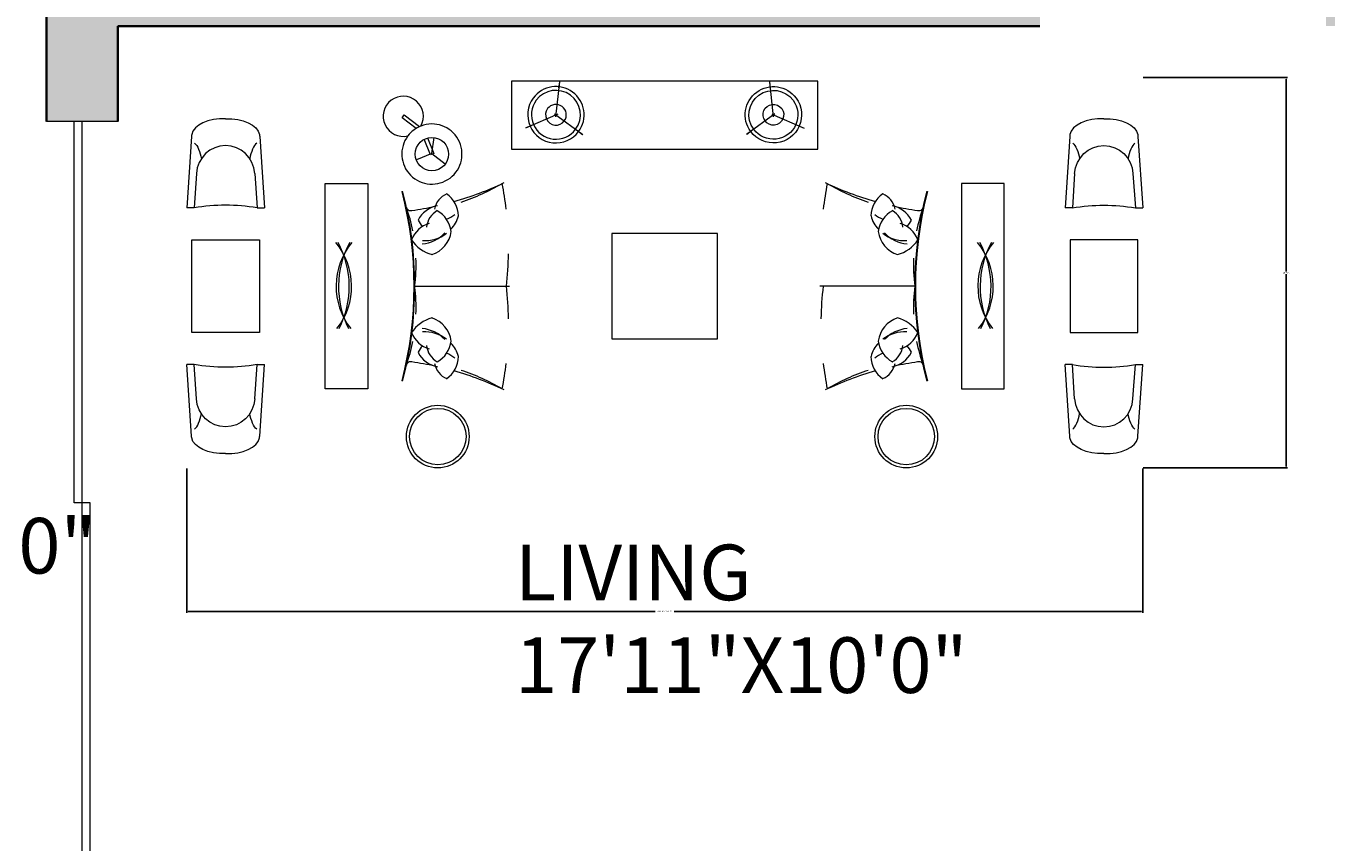
# Model space of a CAD drawing. Units: inches. Extents: x 2540 to 3167, y 3083 to 4007.
# Tile 4 of 15: x 2634 to 2798, y 3313 to 3416. Entities that reach past the tile are written whole.
import ezdxf

# ---------------------------------------------------------------- set-up
doc = ezdxf.new("R2010")
doc.units = ezdxf.units.IN
doc.set_wipeout_variables(frame=1)
for name, color, linetype, lineweight in [('A-ANNO-DIMS', 2, 'Continuous', 18), ('A-AREA-IDEN', 7, 'Continuous', 18), ('A-DOOR', 4, 'Continuous', 18), ('A-FURN', 8, 'Continuous', 13)]:
    doc.layers.add(name, color=color, linetype=linetype, lineweight=lineweight)
doc.layers.add('A-WALL', color=143, linetype='Continuous', lineweight=35, true_color=0x7aafdf)
doc.layers.add('A-WALL-PATT', color=143, linetype='Continuous', lineweight=13, true_color=0x7aafdf)
doc.styles.get("Standard").update_dxf_attribs({"font": 'arial.ttf'})
doc.dimstyles.get("Standard").update_dxf_attribs({"dimtxt": 0.18, "dimasz": 0.18, "dimexe": 0.18, "dimexo": 0.0625, "dimgap": 0.09, "dimtad": 0, "dimtih": 1, "dimtoh": 1, "dimdec": 4, "dimzin": 0, "dimdsep": 46, "dimtxsty": 'Standard', "dimcen": 0.09, "dimadec": 0, "dimazin": 0, "dimtfac": 1, "dimtdec": 4, "dimtofl": 0, "dimtmove": 0, "dimatfit": 3, "dimfxl": 1, "dimtolj": 1, "dimtzin": 0, "dimarcsym": 0})

# ---------------------------------------------------------------- blocks, each defined once
blk = doc.blocks.new('A$C5805318C')
at = {"linetype": 'ByBlock'}
for p, q in [((1718, 2794), (1735, 2817)), ((1718, 2794), (1735, 2817)), ((1735, 2817), (1857, 2723)), ((1735, 2817), (1857, 2723)), ((1829, 2708), (1718, 2794)), ((1829, 2708), (1718, 2794)), ((1945, 2497), (1893, 2622)), ((1945, 2497), (1893, 2622)), ((1919, 2633), (1971, 2508)), ((1919, 2633), (1971, 2508)), ((1955, 2509), (1973, 2636)), ((1955, 2509), (1973, 2636)), ((1955, 2509), (1831, 2459)), ((1955, 2509), (1831, 2459)), ((1971, 2508), (1945, 2497)), ((1971, 2508), (1945, 2497)), ((1955, 2509), (2060, 2427)), ((1955, 2509), (2060, 2427))]:
    blk.add_line(p, q, dxfattribs=at)
for p, q in [((38, 2645), (0, 2075)), ((582, 2645), (620, 2075)), ((7041, 2645), (7003, 2075)), ((7585, 2645), (7623, 2075)), ((77, 2348), (59, 2075)), ((543, 2348), (561, 2075)), ((7080, 2348), (7062, 2075)), ((7545, 2348), (7564, 2075)), ((59, 2075), (0, 2075)), ((561, 2075), (620, 2075)), ((7062, 2075), (7003, 2075)), ((7564, 2075), (7623, 2075)), ((59, 824), (0, 824)), ((38, 254), (0, 824)), ((77, 551), (59, 824)), ((543, 551), (561, 824)), ((561, 824), (620, 824)), ((582, 254), (620, 824)), ((7062, 824), (7003, 824)), ((7041, 254), (7003, 824)), ((7080, 551), (7062, 824)), ((7545, 551), (7564, 824)), ((7564, 824), (7623, 824)), ((7585, 254), (7623, 824))]:
    blk.add_line(p, q)
blk.add_circle((1955, 2504), 133, dxfattribs=at)
blk.add_circle((1955, 2504), 133, dxfattribs=at)
for centre, radius in [((2002, 250), 250), ((2002, 250), 225), ((5737, 250), 250), ((5737, 250), 225)]:
    blk.add_circle(centre, radius)
for centre, radius, start, end in [((1727, 2805), 160, 331.0509, 282.9948), ((1955, 2504), 240, 111.272, 142.7738), ((1955, 2504), 240, 111.272, 142.7738)]:
    blk.add_arc(centre, radius, start, end, dxfattribs=at)
for points in [[(310, 2784), (175, 2792), (54, 2736), (40, 2660), (39, 2654), (38, 2649), (38, 2643)], [(310, 2784), (445, 2792), (566, 2736), (580, 2660), (581, 2654), (582, 2649), (582, 2643)], [(7313, 2784), (7178, 2792), (7057, 2736), (7042, 2660), (7041, 2654), (7041, 2649), (7041, 2643)], [(7313, 2784), (7448, 2792), (7569, 2736), (7583, 2660), (7584, 2654), (7585, 2649), (7585, 2643)], [(310, 116), (175, 108), (54, 163), (40, 240), (39, 245), (38, 251), (38, 256)], [(310, 116), (445, 108), (566, 163), (580, 240), (581, 245), (582, 251), (582, 256)], [(7313, 116), (7178, 108), (7057, 163), (7042, 240), (7041, 245), (7041, 251), (7041, 256)], [(7313, 116), (7448, 108), (7569, 163), (7583, 240), (7584, 245), (7585, 251), (7585, 256)]]:
    blk.add_open_spline(points, degree=3, knots=[0, 0, 0, 0, 1, 1, 1, 2, 2, 2, 2])
for points in [[(62, 2590), (86, 2572), (108, 2522), (117, 2466)], [(310, 2572), (188, 2572), (86, 2474), (77, 2348)], [(543, 2348), (534, 2474), (433, 2572), (310, 2572)], [(558, 2590), (535, 2572), (512, 2522), (503, 2466)], [(7065, 2590), (7088, 2572), (7110, 2522), (7119, 2466)], [(7080, 2348), (7089, 2474), (7190, 2572), (7313, 2572)], [(7313, 2572), (7435, 2572), (7537, 2474), (7545, 2348)], [(7561, 2590), (7537, 2572), (7515, 2522), (7506, 2466)], [(310, 2096), (226, 2096), (142, 2089), (59, 2075)], [(561, 2075), (478, 2089), (394, 2096), (310, 2096)], [(7062, 2075), (7145, 2089), (7229, 2096), (7313, 2096)], [(7313, 2096), (7397, 2096), (7481, 2089), (7564, 2075)], [(310, 804), (226, 804), (142, 810), (59, 824)], [(561, 824), (478, 810), (394, 804), (310, 804)], [(7062, 824), (7145, 810), (7229, 804), (7313, 804)], [(7313, 804), (7397, 804), (7481, 810), (7564, 824)], [(310, 328), (188, 328), (86, 425), (77, 551)], [(543, 551), (534, 425), (433, 328), (310, 328)], [(7080, 551), (7089, 425), (7190, 328), (7313, 328)], [(7313, 328), (7435, 328), (7537, 425), (7545, 551)], [(62, 310), (86, 327), (108, 378), (117, 434)], [(558, 310), (535, 327), (512, 378), (503, 434)], [(7065, 310), (7088, 327), (7110, 378), (7119, 434)], [(7561, 310), (7537, 327), (7515, 378), (7506, 434)]]:
    blk.add_open_spline(points, degree=3)
for points in [[(2561, 3114), (2561, 2514), (5061, 2514), (5061, 3114)], [(1474, 600), (1074, 600), (1074, 2300), (1474, 2300)], [(2575, 1450), (2574, 1519), (2572, 1654), (2567, 1805), (2559, 1944), (2549, 2088), (2540, 2188), (2531, 2276), (2527, 2314), (1674, 2200), (1674, 1450), (1674, 699), (2527, 585), (2531, 623), (2540, 712), (2549, 811), (2559, 956), (2567, 1094), (2572, 1246), (2574, 1380)], [(5048, 1450), (5048, 1519), (5051, 1654), (5056, 1805), (5064, 1944), (5074, 2088), (5083, 2188), (5091, 2276), (5096, 2314), (5949, 2200), (5949, 1450), (5949, 699), (5096, 585), (5091, 623), (5083, 712), (5074, 811), (5064, 956), (5056, 1094), (5051, 1246), (5048, 1380)], [(6149, 600), (6549, 600), (6549, 2300), (6149, 2300)], [(3361, 1000), (4261, 1000), (4261, 1900), (3361, 1900)], [(610, 1050), (10, 1050), (10, 1850), (610, 1850)], [(7013, 1050), (7613, 1050), (7613, 1850), (7013, 1850)]]:
    blk.add_wipeout(points, dxfattribs=at)
for p, q in [((2943, 2802), (2974, 3081)), ((2968, 3032), (2974, 3078)), ((4680, 2802), (4649, 3081)), ((4654, 3032), (4649, 3078)), ((2958, 2823), (2701, 2710)), ((2932, 2826), (3159, 2659)), ((4690, 2826), (4464, 2659)), ((4665, 2823), (4922, 2710)), ((2746, 2730), (2704, 2712)), ((4877, 2730), (4919, 2712)), ((3119, 2688), (3156, 2661)), ((4504, 2688), (4467, 2661))]:
    blk.add_line(p, q, dxfattribs=at)
for p, q in [((1817, 1450), (2575, 1450)), ((5805, 1450), (5048, 1450))]:
    blk.add_line(p, q)
for points in [[(2591, 3084), (2591, 2544), (5031, 2544), (5031, 3084)], [(1444, 630), (1104, 630), (1104, 2270), (1444, 2270)], [(6179, 630), (6519, 630), (6519, 2270), (6179, 2270)], [(3391, 1030), (4231, 1030), (4231, 1870), (3391, 1870)], [(580, 1080), (40, 1080), (40, 1820), (580, 1820)], [(7043, 1080), (7583, 1080), (7583, 1820), (7043, 1820)]]:
    blk.add_lwpolyline(points, close=True, dxfattribs=at)
for centre, radius, start, end in [((1955, 2504), 240, 142.7738, 111.272), ((-1206, 1450), 3024, 345.5057, 14.4943), ((2141, 2032), 169, 113.788, 168.6748), ((1945, 2005), 222, 1.4651, 55.0097), ((1435, 4574), 2546, 285.8776, 295.5087), ((6188, 4574), 2546, 244.4913, 254.1224), ((5678, 2005), 222, 124.9903, 178.5349), ((5482, 2032), 169, 11.3252, 66.212), ((8829, 1450), 3024, 165.5057, 194.4943), ((1785, 2087), 34.6, 193.5328, 287.2771), ((1435, 4574), 2546, 278.134, 282.3755), ((2038, 1878), 217, 100.5196, 152.9581), ((5585, 1878), 217, 27.0419, 79.4804), ((6188, 4574), 2546, 257.6245, 261.866), ((5838, 2087), 34.6, 252.7229, 346.4672), ((2095, 2106), 282, 207.4684, 220.0792), ((2081, 1906), 169, 119.788, 174.6748), ((1889, 1858), 222, 7.4651, 61.0097), ((1947, 2064), 226, 314.9669, 346.4215), ((5676, 2064), 226, 193.5785, 225.0331), ((5734, 1858), 222, 118.9903, 172.5349), ((5542, 1906), 169, 5.3252, 60.212), ((5528, 2106), 282, 319.9208, 332.5316), ((1996, 1742), 217, 106.5196, 158.9581), ((1885, 1917), 226, 288.0023, 352.4215), ((5738, 1917), 226, 187.5785, 251.9977), ((5627, 1742), 217, 21.0419, 73.4804), ((769, 1450), 546, 321.7197, 39.6872), ((1737, 1450), 546, 140.3128, 218.2803), ((564, 1447), 732, 332.7542, 28.6527), ((1942, 1447), 732, 151.3473, 207.2458), ((2028, 1975), 282, 213.4684, 255.3384), ((5595, 1975), 282, 284.6616, 326.5316), ((5885, 1450), 546, 321.7197, 39.6872), ((6854, 1450), 546, 140.3128, 218.2803), ((5681, 1447), 732, 332.7542, 28.6527), ((7058, 1447), 732, 151.3473, 207.2458), ((2028, 924), 282, 104.6616, 146.5316), ((1885, 982), 226, 7.5785, 71.9977), ((5738, 982), 226, 108.0023, 172.4215), ((5595, 924), 282, 33.4684, 75.3384), ((1996, 1158), 217, 201.0419, 253.4804), ((5627, 1158), 217, 286.5196, 338.9581), ((2095, 793), 282, 139.9208, 152.5316), ((2081, 993), 169, 185.3252, 240.212), ((1889, 1041), 222, 298.9903, 352.5349), ((1947, 836), 226, 13.5785, 45.0331), ((5676, 836), 226, 134.9669, 166.4215), ((5734, 1041), 222, 187.4651, 241.0097), ((5542, 993), 169, 299.788, 354.6748), ((5528, 793), 282, 27.4684, 40.0792), ((1785, 813), 34.6, 72.7229, 166.4672), ((1435, -1675), 2546, 77.6245, 81.866), ((2038, 1021), 217, 207.0419, 259.4804), ((2141, 867), 169, 191.3252, 246.212), ((1945, 894), 222, 304.9903, 358.5349), ((5678, 894), 222, 181.4651, 235.0097), ((5482, 867), 169, 293.788, 348.6748), ((5585, 1021), 217, 280.5196, 332.9581), ((6188, -1675), 2546, 98.134, 102.3755), ((5838, 813), 34.6, 13.5328, 107.2771), ((1435, -1675), 2546, 64.4913, 74.1224), ((6188, -1675), 2546, 105.8776, 115.5087)]:
    blk.add_arc(centre, radius, start, end, dxfattribs=at)
for centre, radius, start, end in [((-1206, 1450), 3019, 345.5057, 14.4943), ((1640, 3765), 1733, 288.4757, 300.3241), ((-91, 1753), 2657, 6.7363, 11.1857), ((7714, 1753), 2657, 168.8143, 173.2637), ((5982, 3765), 1733, 239.6759, 251.5243), ((8829, 1450), 3019, 165.5057, 194.4943), ((477, 1627), 1352, 11.274, 19.5243), ((7146, 1627), 1352, 160.4757, 168.726), ((1964, 2245), 282, 292.5627, 307.9208), ((5659, 2245), 282, 232.0792, 247.4373), ((1853, 2068), 282, 275.0195, 316.8895), ((1899, 2095), 282, 266.0508, 307.9208), ((5723, 2095), 282, 232.0792, 273.9492), ((5769, 2068), 282, 223.1105, 264.9805), ((477, 1627), 1352, 352.4802, 2.0119), ((-91, 1753), 2657, 353.4417, 359.0402), ((7146, 1627), 1352, 177.9881, 187.5198), ((477, 1273), 1352, 357.9881, 7.5198), ((-91, 1146), 2657, 0.9598, 6.5583), ((7714, 1146), 2657, 173.4417, 179.0402), ((7146, 1273), 1352, 172.4802, 182.0119), ((1853, 831), 282, 43.1105, 84.9805), ((1899, 804), 282, 52.0792, 93.9492), ((5723, 804), 282, 86.0508, 127.9208), ((5769, 831), 282, 95.0195, 136.8895), ((477, 1273), 1352, 340.4757, 348.726), ((7146, 1273), 1352, 191.274, 199.5243), ((1964, 654), 282, 52.0792, 67.4373), ((-91, 1146), 2657, 348.8143, 353.2637), ((7714, 1146), 2657, 186.7363, 191.1857), ((5659, 654), 282, 112.5627, 127.9208), ((1640, -865), 1733, 59.6759, 71.5243), ((5982, -865), 1733, 108.4757, 120.3241)]:
    blk.add_arc(centre, radius, start, end)
for major_axis, start_param, end_param in [((-159, 159), 3.292387, 6.433979), ((-138, 138), 3.292387, 6.433979), ((-159, 159), 0.150794, 3.292387), ((-138, 138), 0.150794, 3.292387), ((-58.4, 58.4), 0.150794, 3.292387), ((-58.4, 58.4), 3.292387, 6.433979)]:
    blk.add_ellipse((2944, 2817), major_axis=major_axis, ratio=1, start_param=start_param, end_param=end_param, dxfattribs=at)
at = {"linetype": 'ByBlock', "extrusion": (0, 0, -1)}
for major_axis, start_param, end_param in [((159, 159), 3.292387, 6.433979), ((138, 138), 3.292387, 6.433979), ((159, 159), 0.150794, 3.292387), ((138, 138), 0.150794, 3.292387), ((-58.4, 58.4), 4.863183, 8.004776), ((-58.4, 58.4), 1.72159, 4.863183)]:
    blk.add_ellipse((4678, 2817), major_axis=major_axis, ratio=1, start_param=start_param, end_param=end_param, dxfattribs=at)
blk = doc.blocks.new('DOOR-SLIDING-96IN')
for p, q in [((9, 96), (0, 96)), ((3.5, 48), (3.5, 96)), ((4.5, 0), (4.5, 96)), ((5.5, 48), (3.5, 48)), ((5.5, 0), (5.5, 48)), ((9, 0), (0, 0))]:
    blk.add_line(p, q)
blk = doc.blocks.new('*D39')
at = {"layer": 'A-ANNO-DIMS', "color": 0, "lineweight": -2, "transparency": 16777216}
for p, q in [((2654.16, 3360.01), (2654.16, 3341.85)), ((2774.46, 3360.01), (2774.46, 3341.85)), ((2654.34, 3342.03), (2713.12, 3342.03)), ((2774.28, 3342.03), (2715.49, 3342.03))]:
    blk.add_line(p, q, dxfattribs=at)
at = {"layer": 'A-ANNO-DIMS', "color": 0, "transparency": 16777216}
for points in [[(2654.34, 3342.06), (2654.34, 3342), (2654.16, 3342.03)], [(2774.28, 3342.06), (2774.28, 3342), (2774.46, 3342.03)]]:
    blk.add_solid(points, dxfattribs=at)
at = {"layer": 'Defpoints', "color": 0, "transparency": 16777216}
for p in [(2654.16, 3360.08), (2774.46, 3360.08), (2774.46, 3342.03)]:
    blk.add_point(p, dxfattribs=at)
at = {"layer": 'A-ANNO-DIMS', "color": 0, "transparency": 16777216, "insert": (2714.31, 3342.03), "char_height": 0.18, "attachment_point": 5}
blk.add_mtext('\\A1;SEATING 120 TYP.', dxfattribs=at)
blk = doc.blocks.new('*D40')
at = {"layer": 'A-ANNO-DIMS', "color": 0, "lineweight": -2, "transparency": 16777216}
for p, q in [((2774.52, 3409.21), (2792.68, 3409.21)), ((2792.5, 3409.03), (2792.5, 3384.83)), ((2792.5, 3360.26), (2792.5, 3384.46)), ((2774.52, 3360.08), (2792.68, 3360.08))]:
    blk.add_line(p, q, dxfattribs=at)
at = {"layer": 'A-ANNO-DIMS', "color": 0, "transparency": 16777216}
for points in [[(2792.47, 3409.03), (2792.53, 3409.03), (2792.5, 3409.21)], [(2792.47, 3360.26), (2792.53, 3360.26), (2792.5, 3360.08)]]:
    blk.add_solid(points, dxfattribs=at)
at = {"layer": 'Defpoints', "color": 0, "transparency": 16777216}
for p in [(2774.46, 3409.21), (2792.5, 3409.21), (2774.46, 3360.08)]:
    blk.add_point(p, dxfattribs=at)
at = {"layer": 'A-ANNO-DIMS', "color": 0, "transparency": 16777216, "insert": (2792.5, 3384.64), "char_height": 0.18, "attachment_point": 5}
blk.add_mtext('\\A1;49 TYP.', dxfattribs=at)
blk = doc.blocks.new('*D44')
at = {"layer": 'A-ANNO-DIMS', "color": 0, "lineweight": -2, "transparency": 16777216}
for p, q in [((2771.45, 3964.71), (2540.23, 3964.71)), ((2540.41, 3964.53), (2540.41, 3545.4)), ((2540.41, 3125.89), (2540.41, 3545.03)), ((2810.45, 3125.71), (2540.23, 3125.71))]:
    blk.add_line(p, q, dxfattribs=at)
at = {"layer": 'A-ANNO-DIMS', "color": 0, "transparency": 16777216}
for points in [[(2540.38, 3964.53), (2540.44, 3964.53), (2540.41, 3964.71)], [(2540.38, 3125.89), (2540.44, 3125.89), (2540.41, 3125.71)]]:
    blk.add_solid(points, dxfattribs=at)
at = {"layer": 'Defpoints', "color": 0, "transparency": 16777216}
for p in [(2540.41, 3964.71), (2771.51, 3964.71), (2810.51, 3125.71)]:
    blk.add_point(p, dxfattribs=at)
at = {"layer": 'A-ANNO-DIMS', "color": 0, "transparency": 16777216, "insert": (2540.41, 3545.21), "char_height": 0.18, "attachment_point": 5}
blk.add_mtext('\\A1;839', dxfattribs=at)

msp = doc.modelspace()

# ---------------------------------------------------------------- hatches: boundary and pattern name
at = {"layer": 'A-WALL-PATT'}
h = msp.add_hatch(color=256, dxfattribs=at)
h.dxf.hatch_style = 1
h.paths.add_polyline_path([(2805.51, 3803.71), (2800.51, 3803.71), (2800.51, 3799.71), (2621.51, 3799.71), (2621.51, 3823.71), (2612.51, 3823.71), (2612.51, 3794.71), (2636.51, 3794.71), (2636.51, 3782.71), (2645.51, 3782.71), (2645.51, 3794.71), (2805.51, 3794.71)])
h.paths.add_polyline_path([(2810.51, 3564.71), (2868.51, 3564.71), (2868.51, 3627.71), (2872.51, 3627.71), (2872.51, 3636.71), (2864.51, 3636.71), (2864.51, 3674.71), (2797.51, 3674.71), (2797.51, 3669.71), (2801.51, 3669.71), (2801.51, 3628.63), (2806.51, 3628.63), (2806.51, 3669.71), (2859.51, 3669.71), (2859.51, 3573.71), (2806.51, 3573.71), (2806.51, 3598.63), (2801.51, 3598.63), (2801.51, 3549.71), (2645.51, 3549.71), (2645.51, 3573.71), (2636.51, 3573.71), (2636.51, 3516.71), (2645.51, 3516.71), (2645.51, 3540.71), (2801.51, 3540.71), (2801.51, 3504.71), (2801.51, 3500.71), (2806.51, 3500.71), (2806.51, 3504.71), (2859.51, 3504.71), (2859.51, 3420.71), (2806.51, 3420.71), (2806.51, 3470.71), (2801.51, 3470.71), (2801.51, 3420.71), (2797.51, 3420.71), (2797.51, 3415.71), (2864.51, 3415.71), (2864.51, 3453.71), (2868.51, 3453.71), (2868.51, 3513.71), (2810.51, 3513.71)])
h.paths.add_polyline_path([(2645.51, 3415.71), (2761.51, 3415.71), (2761.51, 3420.71), (2645.51, 3420.71), (2645.51, 3444.71), (2636.51, 3444.71), (2636.51, 3403.71), (2645.51, 3403.71)])
h.paths.add_polyline_path([(2645.51, 3307.71), (2636.51, 3307.71), (2636.51, 3295.71), (2612.51, 3295.71), (2612.51, 3149.71), (2645.51, 3149.71), (2645.51, 3158.71), (2621.51, 3158.71), (2621.51, 3290.71), (2801.51, 3290.71), (2801.51, 3286.71), (2806.51, 3286.71), (2806.51, 3295.71), (2645.51, 3295.71)])
h.paths.add_polyline_path([(2762.01, 3158.71), (2746.51, 3158.71), (2746.51, 3240.71), (2750.51, 3240.71), (2750.51, 3245.71), (2741.51, 3245.71), (2741.51, 3158.71), (2717.51, 3158.71), (2717.51, 3149.71), (2762.01, 3149.71)], flags=17)
h.paths.add_polyline_path([(2810.51, 3173.71), (2822.51, 3173.71), (2822.51, 3182.71), (2806.51, 3182.71), (2806.51, 3250.71), (2801.51, 3250.71), (2801.51, 3245.71), (2780.51, 3245.71), (2780.51, 3240.71), (2801.51, 3240.71), (2801.51, 3158.71), (2786.01, 3158.71), (2786.01, 3149.71), (2810.51, 3149.71)])
h.paths.add_polyline_path([(2931.51, 3290.71), (2935.51, 3290.71), (2935.51, 3295.71), (2926.51, 3295.71), (2926.51, 3182.71), (2910.51, 3182.71), (2910.51, 3173.71), (2922.51, 3173.71), (2922.51, 3149.71), (2987.51, 3149.71), (2987.51, 3158.71), (2931.51, 3158.71)])
h.paths.add_polyline_path([(3124.51, 3295.71), (3086.51, 3295.71), (3018.51, 3295.71), (3018.51, 3290.71), (3115.51, 3290.71), (3115.51, 3158.71), (3059.51, 3158.71), (3059.51, 3149.71), (3124.51, 3149.71)])
h.paths.add_polyline_path([(2988.51, 3295.71), (2984.51, 3295.71), (2984.51, 3349.71), (3086.51, 3349.71), (3086.51, 3320.71), (3124.51, 3320.71), (3124.51, 3354.71), (3071.51, 3354.71), (3071.51, 3358.71), (3062.51, 3358.71), (3062.51, 3354.71), (2979.51, 3354.71), (2979.51, 3295.71), (2971.51, 3295.71), (2971.51, 3290.71), (2988.51, 3290.71)])
h.paths.add_polyline_path([(3095.51, 3325.71), (3095.51, 3349.71), (3119.51, 3349.71), (3119.51, 3325.71)], flags=16)
h.paths.add_polyline_path([(3124.51, 3462.71), (3071.51, 3462.71), (3071.51, 3627.71), (3124.51, 3627.71), (3124.51, 3693.71), (3095.51, 3693.71), (3095.51, 3702.71), (3086.51, 3702.71), (3086.51, 3684.71), (3086.51, 3636.71), (2930.51, 3636.71), (2930.51, 3768.71), (2934.51, 3768.71), (2934.51, 3773.71), (2930.51, 3773.71), (2925.51, 3773.71), (2925.51, 3730.71), (2864.51, 3730.71), (2864.51, 3760.71), (2859.51, 3760.71), (2859.51, 3725.71), (2925.51, 3725.71), (2925.51, 3636.71), (2908.51, 3636.71), (2908.51, 3627.71), (3062.51, 3627.71), (3062.51, 3543.71), (2930.51, 3543.71), (2930.51, 3534.71), (2993.51, 3534.71), (2993.51, 3516.71), (3002.51, 3516.71), (3002.51, 3534.71), (3062.51, 3534.71), (3062.51, 3462.71), (3002.51, 3462.71), (3002.51, 3480.71), (2993.51, 3480.71), (2993.51, 3462.71), (2916.51, 3462.71), (2916.51, 3453.71), (2926.51, 3453.71), (2926.51, 3361.71), (2859.51, 3361.71), (2859.51, 3338.71), (2864.51, 3338.71), (2864.51, 3356.71), (2926.51, 3356.71), (2926.51, 3338.71), (2931.51, 3338.71), (2931.51, 3453.71), (3062.51, 3453.71), (3062.51, 3448.21), (3071.51, 3448.21), (3071.51, 3453.71), (3124.51, 3453.71)])

# ---------------------------------------------------------------- linework, layer by layer
at = {"layer": 'A-WALL'}
for p, q in [((2636.51, 3686.71), (2636.51, 3403.71)), ((2645.51, 3415.71), (2761.51, 3415.71)), ((2645.51, 3415.71), (2645.51, 3403.71))]:
    msp.add_line(p, q, dxfattribs=at)

# ---------------------------------------------------------------- block references
at = {"layer": 'A-DOOR'}
msp.add_blockref('DOOR-SLIDING-96IN', (2636.51, 3307.71), dxfattribs=at)

# ---------------------------------------------------------------- texts
at = {"layer": 'A-AREA-IDEN', "char_height": 7, "attachment_point": 1}
for s, width, insert in [('BALCONY\\P10\'4.5"X4\'0"', 97.3161, (2588.51, 3365.46)), ('LIVING\\P17\'11"X10\'0"', 74.1323, (2695.47, 3350.43))]:
    msp.add_mtext_dynamic_manual_height_columns(s, width=width, gutter_width=12.5, heights=[0], dxfattribs=dict(at, insert=insert))

# ---------------------------------------------------------------- next in the draw order: block references
at = {"layer": 'A-FURN', "xscale": 0.0157806756092575, "yscale": 0.0157806756092575, "zscale": 0.0157806756092575}
msp.add_blockref('A$C5805318C', (2654.16, 3360.08), dxfattribs=at)

# ---------------------------------------------------------------- next in the draw order: dimensions: what is measured, and where the dimension line sits
at = {"layer": 'A-ANNO-DIMS'}
dim = msp.add_linear_dim(base=(2540.41, 3964.71), p1=(2810.51, 3125.71), p2=(2771.51, 3964.71), angle=90, dimstyle='Standard', override={"dimdec": 0, "dimlfac": 1, "dimrnd": 0, "dimzin": 0, "dimdsep": 46, "dimlunit": 2}, dxfattribs=at)
dim.commit()
dim.dimension.update_dxf_attribs({"geometry": '*D44', "text_midpoint": (2540.41, 3545.21)})
dim = msp.add_linear_dim(base=(2792.5, 3409.21), p1=(2774.46, 3360.08), p2=(2774.46, 3409.21), angle=90, text='<> TYP.', dimstyle='Standard', override={"dimdec": 0, "dimlfac": 1, "dimrnd": 0, "dimzin": 0, "dimdsep": 46, "dimlunit": 2}, dxfattribs=at)
dim.commit()
dim.dimension.update_dxf_attribs({"geometry": '*D40', "text_midpoint": (2792.5, 3384.64)})
dim = msp.add_linear_dim(base=(2774.46, 3342.03), p1=(2654.16, 3360.08), p2=(2774.46, 3360.08), text='SEATING <> TYP.', dimstyle='Standard', override={"dimdec": 0, "dimlfac": 1, "dimrnd": 0, "dimzin": 0, "dimdsep": 46, "dimlunit": 2}, dxfattribs=at)
dim.commit()
dim.dimension.update_dxf_attribs({"geometry": '*D39', "text_midpoint": (2714.31, 3342.03)})

doc.saveas('drawing.dxf')
